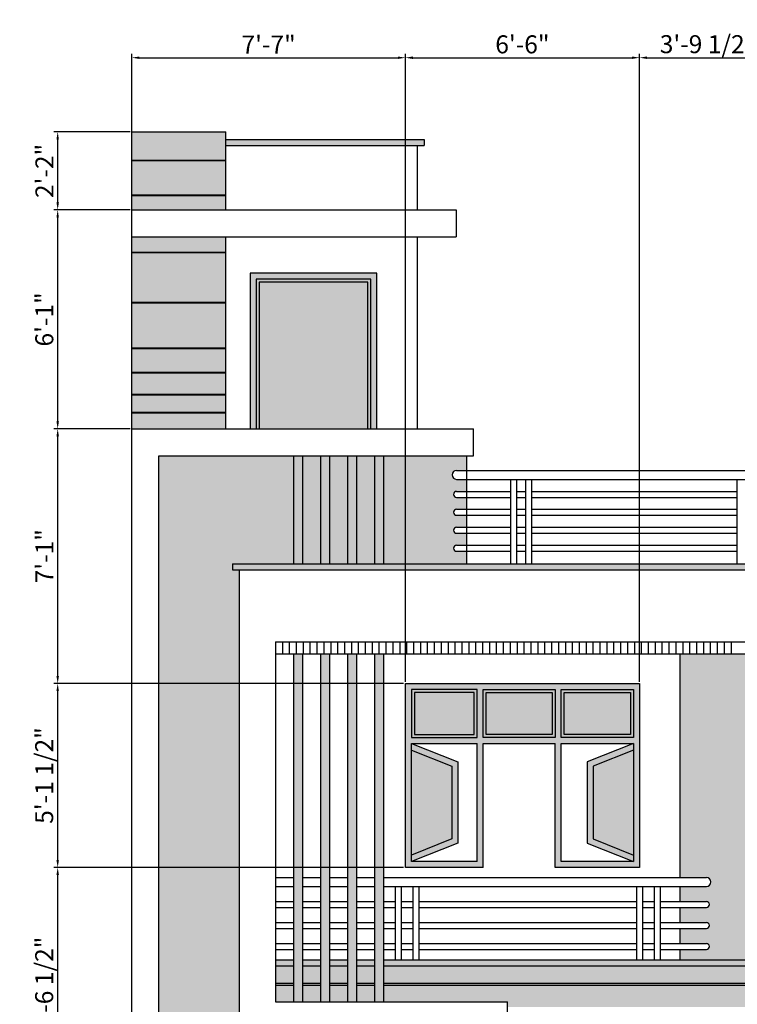
# Model space of a CAD drawing. Units: millimetres. Extents: x 4237 to 5109, y 21391 to 22486.
# Tile 2 of 17: x 4672 to 4911, y 21581 to 21909. Entities that reach past the tile are written whole.
import ezdxf

# ---------------------------------------------------------------- set-up
doc = ezdxf.new("R2010")
doc.units = ezdxf.units.MM
for name, color, linetype, lineweight in [('A-ANNO-DIMS', 2, 'Continuous', 18), ('A-ELEV', 7, 'Continuous', 25), ('A-ELEV-PATT', 252, 'Continuous', 13)]:
    doc.layers.add(name, color=color, linetype=linetype, lineweight=lineweight)
doc.styles.get("Standard").update_dxf_attribs({"font": 'arial.ttf'})
doc.dimstyles.new('ISO-25', dxfattribs={"dimtxt": 6, "dimasz": 2.5, "dimexe": 1.25, "dimexo": 0.625, "dimtad": 1, "dimdec": 1, "dimlunit": 4, "dimtxsty": 'Standard', "dimcen": 2.5, "dimadec": 0, "dimazin": 0, "dimtfac": 1, "dimtdec": 1, "dimtmove": 0, "dimatfit": 3, "dimfxl": 1, "dimarcsym": 0})

# ---------------------------------------------------------------- blocks, each defined once
blk = doc.blocks.new('*D128')
at = {"layer": 'A-ANNO-DIMS', "color": 0, "lineweight": -2, "transparency": 16777216}
for p, q in [((4709.23, 21558.46), (4709.23, 21897.84)), ((4711.73, 21896.59), (4797.95, 21896.59)), ((4800.45, 21688.54), (4800.45, 21897.84))]:
    blk.add_line(p, q, dxfattribs=at)
at = {"layer": 'A-ANNO-DIMS', "color": 0, "transparency": 16777216}
for points in [[(4711.73, 21897), (4711.73, 21896.17), (4709.23, 21896.59)], [(4797.95, 21897), (4797.95, 21896.17), (4800.45, 21896.59)]]:
    blk.add_solid(points, dxfattribs=at)
at = {"layer": 'Defpoints', "color": 0, "transparency": 16777216}
for p in [(4800.45, 21896.59), (4800.45, 21687.91), (4709.23, 21557.84)]:
    blk.add_point(p, dxfattribs=at)
at = {"layer": 'A-ANNO-DIMS', "color": 0, "transparency": 16777216, "insert": (4754.84, 21900.21), "char_height": 6, "attachment_point": 5}
blk.add_mtext('7\'-7"', dxfattribs=at)
blk = doc.blocks.new('*D129')
at = {"layer": 'A-ANNO-DIMS', "color": 0, "lineweight": -2, "transparency": 16777216}
for p, q in [((4800.45, 21688.54), (4800.45, 21897.84)), ((4802.95, 21896.59), (4876.04, 21896.59)), ((4878.54, 21688.54), (4878.54, 21897.84))]:
    blk.add_line(p, q, dxfattribs=at)
at = {"layer": 'A-ANNO-DIMS', "color": 0, "transparency": 16777216}
for points in [[(4802.95, 21897), (4802.95, 21896.17), (4800.45, 21896.59)], [(4876.04, 21897), (4876.04, 21896.17), (4878.54, 21896.59)]]:
    blk.add_solid(points, dxfattribs=at)
at = {"layer": 'Defpoints', "color": 0, "transparency": 16777216}
for p in [(4878.54, 21896.59), (4800.45, 21687.91), (4878.54, 21687.91)]:
    blk.add_point(p, dxfattribs=at)
at = {"layer": 'A-ANNO-DIMS', "color": 0, "transparency": 16777216, "insert": (4839.49, 21900.27), "char_height": 6, "attachment_point": 5}
blk.add_mtext('6\'-6"', dxfattribs=at)
blk = doc.blocks.new('*D130')
at = {"layer": 'A-ANNO-DIMS', "color": 0, "lineweight": -2, "transparency": 16777216}
for p, q in [((4878.54, 21688.54), (4878.54, 21897.84)), ((4881.04, 21896.59), (4921.78, 21896.59)), ((4924.28, 21686.68), (4924.28, 21897.84))]:
    blk.add_line(p, q, dxfattribs=at)
at = {"layer": 'A-ANNO-DIMS', "color": 0, "transparency": 16777216}
for points in [[(4881.04, 21897), (4881.04, 21896.17), (4878.54, 21896.59)], [(4921.78, 21897), (4921.78, 21896.17), (4924.28, 21896.59)]]:
    blk.add_solid(points, dxfattribs=at)
at = {"layer": 'Defpoints', "color": 0, "transparency": 16777216}
for p in [(4924.28, 21896.59), (4878.54, 21687.91), (4924.28, 21686.05)]:
    blk.add_point(p, dxfattribs=at)
at = {"layer": 'A-ANNO-DIMS', "color": 0, "transparency": 16777216, "insert": (4901.41, 21900.32), "char_height": 6, "attachment_point": 5}
blk.add_mtext('3\'-9 1/2"', dxfattribs=at)
blk = doc.blocks.new('*D140')
at = {"layer": 'A-ANNO-DIMS', "color": 0, "lineweight": -2, "transparency": 16777216}
for p, q in [((4799.82, 21626.61), (4683.23, 21626.61)), ((4684.48, 21550.76), (4684.48, 21624.11)), ((4807.6, 21548.26), (4683.23, 21548.26))]:
    blk.add_line(p, q, dxfattribs=at)
at = {"layer": 'A-ANNO-DIMS', "color": 0, "transparency": 16777216}
for points in [[(4684.06, 21624.11), (4684.89, 21624.11), (4684.48, 21626.61)], [(4684.06, 21550.76), (4684.89, 21550.76), (4684.48, 21548.26)]]:
    blk.add_solid(points, dxfattribs=at)
at = {"layer": 'Defpoints', "color": 0, "transparency": 16777216}
for p in [(4684.48, 21626.61), (4800.45, 21626.61), (4808.23, 21548.26)]:
    blk.add_point(p, dxfattribs=at)
at = {"layer": 'A-ANNO-DIMS', "color": 0, "transparency": 16777216, "insert": (4680.75, 21587.44), "char_height": 6, "attachment_point": 5, "rotation": 90}
blk.add_mtext('6\'-6 1/2"', dxfattribs=at)
blk = doc.blocks.new('*D141')
at = {"layer": 'A-ANNO-DIMS', "color": 0, "lineweight": -2, "transparency": 16777216}
for p, q in [((4799.82, 21687.91), (4683.23, 21687.91)), ((4684.48, 21629.11), (4684.48, 21685.41)), ((4799.82, 21626.61), (4683.23, 21626.61))]:
    blk.add_line(p, q, dxfattribs=at)
at = {"layer": 'A-ANNO-DIMS', "color": 0, "transparency": 16777216}
for points in [[(4684.06, 21685.41), (4684.89, 21685.41), (4684.48, 21687.91)], [(4684.06, 21629.11), (4684.89, 21629.11), (4684.48, 21626.61)]]:
    blk.add_solid(points, dxfattribs=at)
at = {"layer": 'Defpoints', "color": 0, "transparency": 16777216}
for p in [(4684.48, 21687.91), (4800.45, 21687.91), (4800.45, 21626.61)]:
    blk.add_point(p, dxfattribs=at)
at = {"layer": 'A-ANNO-DIMS', "color": 0, "transparency": 16777216, "insert": (4680.75, 21657.26), "char_height": 6, "attachment_point": 5, "rotation": 90}
blk.add_mtext('5\'-1 1/2"', dxfattribs=at)
blk = doc.blocks.new('*D142')
at = {"layer": 'A-ANNO-DIMS', "color": 0, "lineweight": -2, "transparency": 16777216}
for p, q in [((4708.6, 21772.84), (4683.23, 21772.84)), ((4684.48, 21690.41), (4684.48, 21770.34)), ((4799.82, 21687.91), (4683.23, 21687.91))]:
    blk.add_line(p, q, dxfattribs=at)
at = {"layer": 'A-ANNO-DIMS', "color": 0, "transparency": 16777216}
for points in [[(4684.06, 21770.34), (4684.89, 21770.34), (4684.48, 21772.84)], [(4684.06, 21690.41), (4684.89, 21690.41), (4684.48, 21687.91)]]:
    blk.add_solid(points, dxfattribs=at)
at = {"layer": 'Defpoints', "color": 0, "transparency": 16777216}
for p in [(4684.48, 21772.84), (4709.23, 21772.84), (4800.45, 21687.91)]:
    blk.add_point(p, dxfattribs=at)
at = {"layer": 'A-ANNO-DIMS', "color": 0, "transparency": 16777216, "insert": (4680.84, 21730.37), "char_height": 6, "attachment_point": 5, "rotation": 90}
blk.add_mtext('7\'-1"', dxfattribs=at)
blk = doc.blocks.new('*D143')
at = {"layer": 'A-ANNO-DIMS', "color": 0, "lineweight": -2, "transparency": 16777216}
for p, q in [((4708.6, 21845.84), (4683.23, 21845.84)), ((4684.48, 21775.34), (4684.48, 21843.34)), ((4708.6, 21772.84), (4683.23, 21772.84))]:
    blk.add_line(p, q, dxfattribs=at)
at = {"layer": 'A-ANNO-DIMS', "color": 0, "transparency": 16777216}
for points in [[(4684.06, 21843.34), (4684.89, 21843.34), (4684.48, 21845.84)], [(4684.06, 21775.34), (4684.89, 21775.34), (4684.48, 21772.84)]]:
    blk.add_solid(points, dxfattribs=at)
at = {"layer": 'Defpoints', "color": 0, "transparency": 16777216}
for p in [(4684.48, 21845.84), (4709.23, 21845.84), (4709.23, 21772.84)]:
    blk.add_point(p, dxfattribs=at)
at = {"layer": 'A-ANNO-DIMS', "color": 0, "transparency": 16777216, "insert": (4680.79, 21809.34), "char_height": 6, "attachment_point": 5, "rotation": 90}
blk.add_mtext('6\'-1"', dxfattribs=at)
blk = doc.blocks.new('*D144')
at = {"layer": 'A-ANNO-DIMS', "color": 0, "lineweight": -2, "transparency": 16777216}
for p, q in [((4708.6, 21871.84), (4683.23, 21871.84)), ((4684.48, 21848.34), (4684.48, 21869.34)), ((4708.6, 21845.84), (4683.23, 21845.84))]:
    blk.add_line(p, q, dxfattribs=at)
at = {"layer": 'A-ANNO-DIMS', "color": 0, "transparency": 16777216}
for points in [[(4684.06, 21869.34), (4684.89, 21869.34), (4684.48, 21871.84)], [(4684.06, 21848.34), (4684.89, 21848.34), (4684.48, 21845.84)]]:
    blk.add_solid(points, dxfattribs=at)
at = {"layer": 'Defpoints', "color": 0, "transparency": 16777216}
for p in [(4684.48, 21871.84), (4709.23, 21871.84), (4709.23, 21845.84)]:
    blk.add_point(p, dxfattribs=at)
at = {"layer": 'A-ANNO-DIMS', "color": 0, "transparency": 16777216, "insert": (4680.84, 21858.84), "char_height": 6, "attachment_point": 5, "rotation": 90}
blk.add_mtext('2\'-2"', dxfattribs=at)

msp = doc.modelspace()

# ---------------------------------------------------------------- hatches: boundary and pattern name
at = {"layer": 'A-ELEV-PATT'}
h = msp.add_hatch(color=256, dxfattribs=at)
h.dxf.hatch_style = 1
h.paths.add_polyline_path([(4740.59, 21871.84), (4709.23, 21871.84), (4709.23, 21862.48), (4740.59, 21862.48)])
h = msp.add_hatch(color=256, dxfattribs=at)
h.dxf.hatch_style = 1
h.paths.add_polyline_path([(4806.71, 21869.32), (4740.59, 21869.32), (4740.59, 21867.32), (4806.71, 21867.32)])
h = msp.add_hatch(color=256, dxfattribs=at)
h.dxf.hatch_style = 1
h.paths.add_polyline_path([(4740.59, 21862.48), (4709.23, 21862.48), (4709.23, 21862.28), (4740.59, 21862.28)])
h = msp.add_hatch(color=256, dxfattribs=at)
h.dxf.hatch_style = 1
h.paths.add_polyline_path([(4740.59, 21862.28), (4709.23, 21862.28), (4709.23, 21850.82), (4740.59, 21850.82)])
h = msp.add_hatch(color=256, dxfattribs=at)
h.dxf.hatch_style = 1
h.paths.add_polyline_path([(4740.59, 21850.82), (4709.23, 21850.82), (4709.23, 21850.62), (4740.59, 21850.62)])
h = msp.add_hatch(color=256, dxfattribs=at)
h.dxf.hatch_style = 1
h.paths.add_polyline_path([(4740.59, 21850.62), (4709.23, 21850.62), (4709.23, 21845.84), (4740.59, 21845.84)])
h = msp.add_hatch(color=256, dxfattribs=at)
h.dxf.hatch_style = 1
h.paths.add_polyline_path([(4740.59, 21836.84), (4709.23, 21836.84), (4709.23, 21831.8), (4740.59, 21831.8)])
h = msp.add_hatch(color=256, dxfattribs=at)
h.dxf.hatch_style = 1
h.paths.add_polyline_path([(4740.59, 21831.8), (4709.23, 21831.8), (4709.23, 21831.6), (4740.59, 21831.6)])
h = msp.add_hatch(color=256, dxfattribs=at)
h.dxf.hatch_style = 1
h.paths.add_polyline_path([(4740.59, 21831.6), (4709.23, 21831.6), (4709.23, 21815.08), (4740.59, 21815.08)])
h = msp.add_hatch(color=256, dxfattribs=at)
h.dxf.hatch_style = 1
h.paths.add_polyline_path([(4740.59, 21831.6), (4709.23, 21831.6), (4709.23, 21815.08), (4740.59, 21815.08)])
h = msp.add_hatch(color=256, dxfattribs=at)
h.dxf.hatch_style = 1
h.paths.add_polyline_path([(4790.91, 21824.78), (4748.66, 21824.78), (4748.66, 21772.84), (4750.66, 21772.84), (4750.66, 21822.78), (4788.91, 21822.78), (4788.91, 21772.84), (4790.91, 21772.84)])
h = msp.add_hatch(color=256, dxfattribs=at)
h.dxf.hatch_style = 1
h.paths.add_polyline_path([(4788.91, 21822.78), (4750.66, 21822.78), (4750.66, 21772.84), (4751.66, 21772.84), (4751.66, 21821.78), (4787.91, 21821.78), (4787.91, 21772.84), (4788.91, 21772.84)])
h = msp.add_hatch(color=256, dxfattribs=at)
h.dxf.hatch_style = 1
h.set_gradient(color1=(122, 175, 223), color2=(215, 235, 210), name='INVCYLINDER')
h.paths.add_polyline_path([(4787.91, 21821.78), (4751.66, 21821.78), (4751.66, 21772.84), (4787.91, 21772.84)])
h = msp.add_hatch(color=256, dxfattribs=at)
h.dxf.hatch_style = 1
h.paths.add_polyline_path([(4740.59, 21815.08), (4709.23, 21815.08), (4709.23, 21814.88), (4740.59, 21814.88)])
h = msp.add_hatch(color=256, dxfattribs=at)
h.dxf.hatch_style = 1
h.paths.add_polyline_path([(4740.59, 21814.88), (4709.23, 21814.88), (4709.23, 21799.83), (4740.59, 21799.83)])
h = msp.add_hatch(color=256, dxfattribs=at)
h.dxf.hatch_style = 1
h.paths.add_polyline_path([(4740.59, 21799.83), (4709.23, 21799.83), (4709.23, 21799.63), (4740.59, 21799.63)])
h = msp.add_hatch(color=256, dxfattribs=at)
h.dxf.hatch_style = 1
h.paths.add_polyline_path([(4740.59, 21799.63), (4709.23, 21799.63), (4709.23, 21791.76), (4740.59, 21791.76)])
h = msp.add_hatch(color=256, dxfattribs=at)
h.dxf.hatch_style = 1
h.paths.add_polyline_path([(4740.59, 21791.76), (4709.23, 21791.76), (4709.23, 21791.56), (4740.59, 21791.56)])
h = msp.add_hatch(color=256, dxfattribs=at)
h.dxf.hatch_style = 1
h.paths.add_polyline_path([(4740.59, 21791.56), (4709.23, 21791.56), (4709.23, 21784.38), (4740.59, 21784.38)])
h = msp.add_hatch(color=256, dxfattribs=at)
h.dxf.hatch_style = 1
h.paths.add_polyline_path([(4740.59, 21784.38), (4709.23, 21784.38), (4709.23, 21784.18), (4740.59, 21784.18)])
h = msp.add_hatch(color=256, dxfattribs=at)
h.dxf.hatch_style = 1
h.paths.add_polyline_path([(4740.59, 21784.18), (4709.23, 21784.18), (4709.23, 21778.39), (4740.59, 21778.39)])
h = msp.add_hatch(color=256, dxfattribs=at)
h.dxf.hatch_style = 1
h.paths.add_polyline_path([(4740.59, 21778.39), (4709.23, 21778.39), (4709.23, 21778.19), (4740.59, 21778.19)])
h = msp.add_hatch(color=256, dxfattribs=at)
h.dxf.hatch_style = 1
h.paths.add_polyline_path([(4740.59, 21778.19), (4709.23, 21778.19), (4709.23, 21772.84), (4740.59, 21772.84)])
h = msp.add_hatch(color=256, dxfattribs=at)
h.dxf.hatch_style = 1
h.paths.add_polyline_path([(4763.12, 21763.84), (4718.23, 21763.84), (4718.23, 21557.84), (4745.15, 21557.84), (4745.15, 21725.84), (4742.84, 21725.84), (4742.84, 21727.84), (4763.12, 21727.84)])
h = msp.add_hatch(color=256, dxfattribs=at)
h.dxf.hatch_style = 1
h.paths.add_polyline_path([(4766.12, 21763.84), (4763.12, 21763.84), (4763.12, 21727.84), (4766.12, 21727.84)])
h = msp.add_hatch(color=256, dxfattribs=at)
h.dxf.hatch_style = 1
h.paths.add_polyline_path([(4772.12, 21763.84), (4766.12, 21763.84), (4766.12, 21727.84), (4772.12, 21727.84)])
h = msp.add_hatch(color=256, dxfattribs=at)
h.dxf.hatch_style = 1
h.paths.add_polyline_path([(4775.12, 21763.84), (4772.12, 21763.84), (4772.12, 21727.84), (4775.12, 21727.84)])
h = msp.add_hatch(color=256, dxfattribs=at)
h.dxf.hatch_style = 1
h.paths.add_polyline_path([(4781.12, 21763.84), (4775.12, 21763.84), (4775.12, 21727.84), (4781.12, 21727.84)])
h = msp.add_hatch(color=256, dxfattribs=at)
h.dxf.hatch_style = 1
h.paths.add_polyline_path([(4784.12, 21763.84), (4781.12, 21763.84), (4781.12, 21727.84), (4784.12, 21727.84)])
h = msp.add_hatch(color=256, dxfattribs=at)
h.dxf.hatch_style = 1
h.paths.add_polyline_path([(4790.12, 21763.84), (4784.12, 21763.84), (4784.12, 21727.84), (4790.12, 21727.84)])
h = msp.add_hatch(color=256, dxfattribs=at)
h.dxf.hatch_style = 1
h.paths.add_polyline_path([(4793.12, 21763.84), (4790.12, 21763.84), (4790.12, 21727.84), (4793.12, 21727.84)])
h = msp.add_hatch(color=256, dxfattribs=at)
h.dxf.hatch_style = 1
h.paths.add_polyline_path([(4817.54, 21740.01), (4820.82, 21740.01), (4820.82, 21744.01), (4817.54, 21744.01, -1), (4817.54, 21746.01), (4820.82, 21746.01), (4820.82, 21750.01), (4817.54, 21750.01, -1), (4817.54, 21752.01), (4820.82, 21752.01), (4820.82, 21756.01), (4817.54, 21756.01, -1), (4817.54, 21759.01), (4820.82, 21759.01), (4820.82, 21763.84), (4793.12, 21763.84), (4793.12, 21727.84), (4820.82, 21727.84), (4820.82, 21732.01), (4817.54, 21732.01, -1), (4817.54, 21734.01), (4820.82, 21734.01), (4820.82, 21738.01), (4817.54, 21738.01, -1)])
h = msp.add_hatch(color=256, dxfattribs=at)
h.dxf.hatch_style = 1
h.paths.add_polyline_path([(5017.14, 21727.84), (4742.84, 21727.84), (4742.84, 21725.84), (5017.14, 21725.84)])
h = msp.add_hatch(color=256, dxfattribs=at)
h.dxf.hatch_style = 1
h.paths.add_polyline_path([(4766.12, 21697.84), (4763.12, 21697.84), (4763.12, 21581.84), (4766.12, 21581.84)])
h = msp.add_hatch(color=256, dxfattribs=at)
h.dxf.hatch_style = 1
h.paths.add_polyline_path([(4775.12, 21697.84), (4772.12, 21697.84), (4772.12, 21581.84), (4775.12, 21581.84)])
h = msp.add_hatch(color=256, dxfattribs=at)
h.dxf.hatch_style = 1
h.paths.add_polyline_path([(4784.12, 21697.84), (4781.12, 21697.84), (4781.12, 21581.84), (4784.12, 21581.84)])
h = msp.add_hatch(color=256, dxfattribs=at)
h.dxf.hatch_style = 1
h.paths.add_polyline_path([(4793.12, 21697.84), (4790.12, 21697.84), (4790.12, 21581.84), (4793.12, 21581.84)])
h = msp.add_hatch(color=256, dxfattribs=at)
h.dxf.hatch_style = 1
h.paths.add_polyline_path([(4978.93, 21697.84), (4892.07, 21697.84), (4892.07, 21623.26), (4900.89, 21623.26, -1), (4900.89, 21620.26), (4892.07, 21620.26), (4892.07, 21615.26), (4900.89, 21615.26, -1), (4900.89, 21613.26), (4892.07, 21613.26), (4892.07, 21608.26), (4900.89, 21608.26, -1), (4900.89, 21606.26), (4892.07, 21606.26), (4892.07, 21601.26), (4900.89, 21601.26, -1), (4900.89, 21599.26), (4892.07, 21599.26), (4892.07, 21595.84), (4978.93, 21595.84)])
h.paths.add_polyline_path([(4924.28, 21686.05), (4966.23, 21686.05), (4966.23, 21613.83), (4924.28, 21613.83)], flags=16)
h.paths.add_polyline_path([(4926.28, 21661.68), (4940.28, 21661.68), (4940.28, 21615.68), (4926.28, 21615.68)], flags=0)
h.paths.add_polyline_path([(4942.28, 21661.68), (4964.23, 21661.68), (4964.23, 21615.68), (4942.28, 21615.68)], flags=0)
h.paths.add_polyline_path([(4926.28, 21663.68), (4926.28, 21684.05), (4964.23, 21684.05), (4964.23, 21663.68)], flags=0)
h.paths.add_polyline_path([(4927.28, 21664.68), (4927.28, 21683.05), (4963.23, 21683.05), (4963.23, 21664.68)], flags=0)
h = msp.add_hatch(color=256, dxfattribs=at)
h.dxf.hatch_style = 1
h.paths.add_polyline_path([(4826.45, 21667.91), (4850.45, 21667.91), (4850.45, 21626.61), (4878.54, 21626.61), (4878.54, 21687.91), (4800.45, 21687.91), (4800.45, 21626.61), (4826.45, 21626.61)])
h.paths.add_polyline_path([(4802.45, 21628.61), (4802.45, 21667.91), (4824.45, 21667.91), (4824.45, 21628.61)], flags=16)
h.paths.add_polyline_path([(4802.45, 21669.91), (4802.45, 21685.91), (4824.45, 21685.91), (4824.45, 21669.91)], flags=16)
h.paths.add_polyline_path([(4803.45, 21670.91), (4803.45, 21684.91), (4823.45, 21684.91), (4823.45, 21670.91)], flags=0)
h.paths.add_polyline_path([(4826.45, 21669.91), (4826.45, 21685.91), (4850.45, 21685.91), (4850.45, 21669.91)], flags=16)
h.paths.add_polyline_path([(4827.45, 21670.91), (4827.45, 21684.91), (4849.45, 21684.91), (4849.45, 21670.91)], flags=0)
h.paths.add_polyline_path([(4852.45, 21628.61), (4852.45, 21667.91), (4876.54, 21667.91), (4876.54, 21628.61)], flags=16)
h.paths.add_polyline_path([(4852.45, 21669.91), (4852.45, 21685.91), (4876.54, 21685.91), (4876.54, 21669.91)], flags=16)
h.paths.add_polyline_path([(4853.45, 21670.91), (4853.45, 21684.91), (4875.54, 21684.91), (4875.54, 21670.91)], flags=0)
h = msp.add_hatch(color=256, dxfattribs=at)
h.dxf.hatch_style = 1
h.set_gradient(color1=(122, 175, 223), color2=(215, 235, 210), name='CYLINDER')
h.paths.add_polyline_path([(4824.45, 21685.91), (4802.45, 21685.91), (4802.45, 21669.91), (4824.45, 21669.91)])
h.paths.add_polyline_path([(4823.45, 21684.91), (4823.45, 21670.91), (4803.45, 21670.91), (4803.45, 21684.91)], flags=16)
h = msp.add_hatch(color=256, dxfattribs=at)
h.dxf.hatch_style = 1
h.set_gradient(color1=(122, 175, 223), color2=(215, 235, 210), name='HEMISPHERICAL')
h.paths.add_polyline_path([(4823.45, 21684.91), (4803.45, 21684.91), (4803.45, 21670.91), (4823.45, 21670.91)])
h = msp.add_hatch(color=256, dxfattribs=at)
h.dxf.hatch_style = 1
h.set_gradient(color1=(122, 175, 223), color2=(215, 235, 210), name='CYLINDER')
h.paths.add_polyline_path([(4850.45, 21685.91), (4826.45, 21685.91), (4826.45, 21669.91), (4850.45, 21669.91)])
h.paths.add_polyline_path([(4849.45, 21684.91), (4849.45, 21670.91), (4827.45, 21670.91), (4827.45, 21684.91)], flags=16)
h = msp.add_hatch(color=256, dxfattribs=at)
h.dxf.hatch_style = 1
h.set_gradient(color1=(122, 175, 223), color2=(215, 235, 210), name='HEMISPHERICAL')
h.paths.add_polyline_path([(4849.45, 21684.91), (4827.45, 21684.91), (4827.45, 21670.91), (4849.45, 21670.91)])
h = msp.add_hatch(color=256, dxfattribs=at)
h.dxf.hatch_style = 1
h.set_gradient(color1=(122, 175, 223), color2=(215, 235, 210), name='CYLINDER')
h.paths.add_polyline_path([(4876.54, 21685.91), (4852.45, 21685.91), (4852.45, 21669.91), (4876.54, 21669.91)])
h.paths.add_polyline_path([(4875.54, 21684.91), (4875.54, 21670.91), (4853.45, 21670.91), (4853.45, 21684.91)], flags=16)
h = msp.add_hatch(color=256, dxfattribs=at)
h.dxf.hatch_style = 1
h.set_gradient(color1=(122, 175, 223), color2=(215, 235, 210), name='HEMISPHERICAL')
h.paths.add_polyline_path([(4875.54, 21684.91), (4853.45, 21684.91), (4853.45, 21670.91), (4875.54, 21670.91)])
h = msp.add_hatch(color=256, dxfattribs=at)
h.dxf.hatch_style = 1
h.paths.add_polyline_path([(4817.91, 21661.78), (4802.45, 21667.91), (4802.45, 21665.76), (4815.91, 21660.43), (4815.91, 21636.1), (4802.45, 21630.76), (4802.45, 21628.61), (4817.91, 21634.74)])
h = msp.add_hatch(color=256, dxfattribs=at)
h.dxf.hatch_style = 1
h.paths.add_polyline_path([(4863.07, 21660.43), (4876.54, 21665.76), (4876.54, 21667.91), (4861.07, 21661.78), (4861.07, 21634.74), (4876.54, 21628.61), (4876.54, 21630.76), (4863.07, 21636.1)])
h = msp.add_hatch(color=256, dxfattribs=at)
h.dxf.hatch_style = 1
h.set_gradient(color1=(122, 175, 223), color2=(215, 235, 210), name='CYLINDER')
h.paths.add_polyline_path([(4815.91, 21660.43), (4802.45, 21665.76), (4802.45, 21630.76), (4815.91, 21636.1)])
h = msp.add_hatch(color=256, dxfattribs=at)
h.dxf.hatch_style = 1
h.set_gradient(color1=(122, 175, 223), color2=(215, 235, 210), name='CYLINDER')
h.paths.add_polyline_path([(4876.54, 21665.76), (4863.07, 21660.43), (4863.07, 21636.1), (4876.54, 21630.76)])
h = msp.add_hatch(color=256, dxfattribs=at)
h.dxf.hatch_style = 1
h.paths.add_polyline_path([(5033.17, 21598.15), (5022.76, 21598.15), (5022.76, 21595.84), (5025.55, 21595.84), (5025.55, 21593.84), (4991.17, 21593.84), (4991.17, 21595.84), (4997.2, 21595.84), (4997.2, 21598.15), (4978.93, 21598.15), (4978.93, 21595.84), (4981.84, 21595.84), (4981.84, 21593.84), (4793.12, 21593.84), (4793.12, 21588.01), (5033.17, 21588.01)])
h = msp.add_hatch(color=256, dxfattribs=at)
h.dxf.hatch_style = 1
h.paths.add_polyline_path([(4763.12, 21595.84), (4757.12, 21595.84), (4757.12, 21593.84), (4763.12, 21593.84)])
h = msp.add_hatch(color=256, dxfattribs=at)
h.dxf.hatch_style = 1
h.paths.add_polyline_path([(4772.12, 21595.84), (4766.12, 21595.84), (4766.12, 21593.84), (4772.12, 21593.84)])
h = msp.add_hatch(color=256, dxfattribs=at)
h.dxf.hatch_style = 1
h.paths.add_polyline_path([(4781.12, 21595.84), (4775.12, 21595.84), (4775.12, 21593.84), (4781.12, 21593.84)])
h = msp.add_hatch(color=256, dxfattribs=at)
h.dxf.hatch_style = 1
h.paths.add_polyline_path([(4790.12, 21595.84), (4784.12, 21595.84), (4784.12, 21593.84), (4790.12, 21593.84)])
h = msp.add_hatch(color=256, dxfattribs=at)
h.dxf.hatch_style = 1
h.paths.add_polyline_path([(4981.84, 21595.84), (4793.12, 21595.84), (4793.12, 21593.84), (4981.84, 21593.84)])
h = msp.add_hatch(color=256, dxfattribs=at)
h.dxf.hatch_style = 1
h.paths.add_polyline_path([(4763.12, 21593.84), (4757.12, 21593.84), (4757.12, 21588.01), (4763.12, 21588.01)])
h = msp.add_hatch(color=256, dxfattribs=at)
h.dxf.hatch_style = 1
h.paths.add_polyline_path([(4772.12, 21593.84), (4766.12, 21593.84), (4766.12, 21588.01), (4772.12, 21588.01)])
h = msp.add_hatch(color=256, dxfattribs=at)
h.dxf.hatch_style = 1
h.paths.add_polyline_path([(4781.12, 21593.84), (4775.12, 21593.84), (4775.12, 21588.01), (4781.12, 21588.01)])
h = msp.add_hatch(color=256, dxfattribs=at)
h.dxf.hatch_style = 1
h.paths.add_polyline_path([(4790.12, 21593.84), (4784.12, 21593.84), (4784.12, 21588.01), (4790.12, 21588.01)])
h = msp.add_hatch(color=256, dxfattribs=at)
h.dxf.hatch_style = 1
h.paths.add_polyline_path([(4763.12, 21588.01), (4757.12, 21588.01), (4757.12, 21587.38), (4763.12, 21587.38)])
h = msp.add_hatch(color=256, dxfattribs=at)
h.dxf.hatch_style = 1
h.paths.add_polyline_path([(4772.12, 21588.01), (4766.12, 21588.01), (4766.12, 21587.38), (4772.12, 21587.38)])
h = msp.add_hatch(color=256, dxfattribs=at)
h.dxf.hatch_style = 1
h.paths.add_polyline_path([(4781.12, 21588.01), (4775.12, 21588.01), (4775.12, 21587.38), (4781.12, 21587.38)])
h = msp.add_hatch(color=256, dxfattribs=at)
h.dxf.hatch_style = 1
h.paths.add_polyline_path([(4790.12, 21588.01), (4784.12, 21588.01), (4784.12, 21587.38), (4790.12, 21587.38)])
h = msp.add_hatch(color=256, dxfattribs=at)
h.dxf.hatch_style = 1
h.paths.add_polyline_path([(5033.17, 21588.01), (4793.12, 21588.01), (4793.12, 21587.38), (5033.17, 21587.38)])
h = msp.add_hatch(color=256, dxfattribs=at)
h.dxf.hatch_style = 1
h.paths.add_polyline_path([(4763.12, 21587.38), (4757.12, 21587.38), (4757.12, 21581.84), (4763.12, 21581.84)])
h = msp.add_hatch(color=256, dxfattribs=at)
h.dxf.hatch_style = 1
h.paths.add_polyline_path([(4772.12, 21587.38), (4766.12, 21587.38), (4766.12, 21581.84), (4772.12, 21581.84)])
h = msp.add_hatch(color=256, dxfattribs=at)
h.dxf.hatch_style = 1
h.paths.add_polyline_path([(4781.12, 21587.38), (4775.12, 21587.38), (4775.12, 21581.84), (4781.12, 21581.84)])
h = msp.add_hatch(color=256, dxfattribs=at)
h.dxf.hatch_style = 1
h.paths.add_polyline_path([(4790.12, 21587.38), (4784.12, 21587.38), (4784.12, 21581.84), (4790.12, 21581.84)])
h = msp.add_hatch(color=256, dxfattribs=at)
h.dxf.hatch_style = 1
h.paths.add_polyline_path([(5033.17, 21587.38), (4793.12, 21587.38), (4793.12, 21581.84), (4834.56, 21581.84), (4834.56, 21580.12), (5033.17, 21580.12)])

# ---------------------------------------------------------------- linework, layer by layer
at = {"layer": 'A-ELEV'}
for p, q in [((4709.23, 21425.84), (4709.23, 21871.84)), ((4709.23, 21871.84), (4740.59, 21871.84)), ((4740.59, 21845.84), (4740.59, 21871.84)), ((4740.59, 21869.32), (4806.71, 21869.32)), ((4740.59, 21867.32), (4806.71, 21867.32)), ((4804.53, 21845.84), (4804.53, 21867.32)), ((4806.71, 21869.32), (4806.71, 21867.32)), ((4709.23, 21862.48), (4740.59, 21862.48)), ((4709.23, 21862.28), (4740.59, 21862.28)), ((4709.23, 21850.82), (4740.59, 21850.82)), ((4709.23, 21850.62), (4740.59, 21850.62)), ((4709.23, 21845.84), (4817.34, 21845.84)), ((4817.34, 21845.84), (4817.34, 21836.84)), ((4709.23, 21836.84), (4817.34, 21836.84)), ((4740.59, 21772.84), (4740.59, 21836.84)), ((4804.53, 21772.84), (4804.53, 21836.84)), ((4709.23, 21831.8), (4740.59, 21831.8)), ((4709.23, 21831.6), (4740.59, 21831.6)), ((4709.23, 21815.08), (4740.59, 21815.08)), ((4709.23, 21814.88), (4740.59, 21814.88)), ((4709.23, 21799.83), (4740.59, 21799.83)), ((4709.23, 21799.63), (4740.59, 21799.63)), ((4709.23, 21791.76), (4740.59, 21791.76)), ((4709.23, 21791.56), (4740.59, 21791.56)), ((4709.23, 21784.38), (4740.59, 21784.38)), ((4709.23, 21784.18), (4740.59, 21784.18)), ((4709.23, 21778.39), (4740.59, 21778.39)), ((4709.23, 21778.19), (4740.59, 21778.19)), ((4709.23, 21772.84), (4823.22, 21772.84)), ((4823.22, 21763.84), (4823.22, 21772.84)), ((4718.23, 21557.84), (4718.23, 21763.84)), ((4718.23, 21763.84), (4823.22, 21763.84)), ((4763.12, 21763.84), (4763.12, 21727.84)), ((4766.12, 21763.84), (4766.12, 21727.84)), ((4772.12, 21763.84), (4772.12, 21727.84)), ((4775.12, 21763.84), (4775.12, 21727.84)), ((4781.12, 21763.84), (4781.12, 21727.84)), ((4784.12, 21763.84), (4784.12, 21727.84)), ((4790.12, 21763.84), (4790.12, 21727.84)), ((4793.12, 21763.84), (4793.12, 21727.84)), ((4820.82, 21763.84), (4820.82, 21727.84)), ((4817.54, 21759.01), (4931.32, 21759.01)), ((4817.54, 21756.01), (4931.32, 21756.01)), ((4835.52, 21756.01), (4835.52, 21727.84)), ((4837.52, 21756.01), (4837.52, 21727.84)), ((4840.56, 21756.01), (4840.56, 21727.84)), ((4842.56, 21756.01), (4842.56, 21727.84)), ((4910.97, 21756.01), (4910.97, 21727.84)), ((4817.54, 21752.01), (4835.52, 21752.01)), ((4817.54, 21750.01), (4835.52, 21750.01)), ((4837.52, 21752.01), (4840.56, 21752.01)), ((4837.52, 21750.01), (4840.56, 21750.01)), ((4842.56, 21752.01), (4910.97, 21752.01)), ((4842.56, 21750.01), (4910.97, 21750.01)), ((4817.54, 21746.01), (4835.52, 21746.01)), ((4837.52, 21746.01), (4840.56, 21746.01)), ((4842.56, 21746.01), (4910.97, 21746.01)), ((4817.54, 21744.01), (4835.52, 21744.01)), ((4837.52, 21744.01), (4840.56, 21744.01)), ((4842.56, 21744.01), (4910.97, 21744.01)), ((4817.54, 21740.01), (4835.52, 21740.01)), ((4837.52, 21740.01), (4840.56, 21740.01)), ((4842.56, 21740.01), (4910.97, 21740.01)), ((4817.54, 21738.01), (4835.52, 21738.01)), ((4837.52, 21738.01), (4840.56, 21738.01)), ((4842.56, 21738.01), (4910.97, 21738.01)), ((4817.54, 21734.01), (4835.52, 21734.01)), ((4837.52, 21734.01), (4840.56, 21734.01)), ((4842.56, 21734.01), (4910.97, 21734.01)), ((4817.54, 21732.01), (4835.52, 21732.01)), ((4837.52, 21732.01), (4840.56, 21732.01)), ((4842.56, 21732.01), (4910.97, 21732.01)), ((4742.84, 21727.84), (5017.14, 21727.84)), ((4742.84, 21727.84), (4742.84, 21725.84)), ((4742.84, 21725.84), (5017.14, 21725.84)), ((4745.15, 21557.84), (4745.15, 21725.84)), ((4757.12, 21701.84), (5017.14, 21701.84)), ((4757.12, 21701.84), (4757.12, 21581.84)), ((4759.42, 21701.84), (4759.42, 21697.84)), ((4761.72, 21701.84), (4761.72, 21697.84)), ((4764.02, 21701.84), (4764.02, 21697.84)), ((4766.33, 21701.84), (4766.33, 21697.84)), ((4768.63, 21701.84), (4768.63, 21697.84)), ((4770.93, 21701.84), (4770.93, 21697.84)), ((4773.23, 21701.84), (4773.23, 21697.84)), ((4775.54, 21701.84), (4775.54, 21697.84)), ((4777.84, 21701.84), (4777.84, 21697.84)), ((4780.14, 21701.84), (4780.14, 21697.84)), ((4782.44, 21701.84), (4782.44, 21697.84)), ((4784.75, 21701.84), (4784.75, 21697.84)), ((4787.05, 21701.84), (4787.05, 21697.84)), ((4789.35, 21701.84), (4789.35, 21697.84)), ((4791.65, 21701.84), (4791.65, 21697.84)), ((4793.96, 21701.84), (4793.96, 21697.84)), ((4796.26, 21701.84), (4796.26, 21697.84)), ((4798.56, 21701.84), (4798.56, 21697.84)), ((4800.86, 21701.84), (4800.86, 21697.84)), ((4803.16, 21701.84), (4803.16, 21697.84)), ((4805.47, 21701.84), (4805.47, 21697.84)), ((4807.77, 21701.84), (4807.77, 21697.84)), ((4810.07, 21701.84), (4810.07, 21697.84)), ((4812.37, 21701.84), (4812.37, 21697.84)), ((4814.68, 21701.84), (4814.68, 21697.84)), ((4816.98, 21701.84), (4816.98, 21697.84)), ((4819.28, 21701.84), (4819.28, 21697.84)), ((4821.58, 21701.84), (4821.58, 21697.84)), ((4823.89, 21701.84), (4823.89, 21697.84)), ((4826.19, 21701.84), (4826.19, 21697.84)), ((4828.49, 21701.84), (4828.49, 21697.84)), ((4830.79, 21701.84), (4830.79, 21697.84)), ((4833.1, 21701.84), (4833.1, 21697.84)), ((4835.4, 21701.84), (4835.4, 21697.84)), ((4837.7, 21701.84), (4837.7, 21697.84)), ((4840, 21701.84), (4840, 21697.84)), ((4842.31, 21701.84), (4842.31, 21697.84)), ((4844.61, 21701.84), (4844.61, 21697.84)), ((4846.91, 21701.84), (4846.91, 21697.84)), ((4849.21, 21701.84), (4849.21, 21697.84)), ((4851.51, 21701.84), (4851.51, 21697.84)), ((4853.82, 21701.84), (4853.82, 21697.84)), ((4856.12, 21701.84), (4856.12, 21697.84)), ((4858.42, 21701.84), (4858.42, 21697.84)), ((4860.72, 21701.84), (4860.72, 21697.84)), ((4863.03, 21701.84), (4863.03, 21697.84)), ((4865.33, 21701.84), (4865.33, 21697.84)), ((4867.63, 21701.84), (4867.63, 21697.84)), ((4869.93, 21701.84), (4869.93, 21697.84)), ((4872.24, 21701.84), (4872.24, 21697.84)), ((4874.54, 21701.84), (4874.54, 21697.84)), ((4876.84, 21701.84), (4876.84, 21697.84)), ((4879.14, 21701.84), (4879.14, 21697.84)), ((4881.45, 21701.84), (4881.45, 21697.84)), ((4883.75, 21701.84), (4883.75, 21697.84)), ((4886.05, 21701.84), (4886.05, 21697.84)), ((4888.35, 21701.84), (4888.35, 21697.84)), ((4890.66, 21701.84), (4890.66, 21697.84)), ((4892.96, 21701.84), (4892.96, 21697.84)), ((4895.26, 21701.84), (4895.26, 21697.84)), ((4897.56, 21701.84), (4897.56, 21697.84)), ((4899.86, 21701.84), (4899.86, 21697.84)), ((4902.17, 21701.84), (4902.17, 21697.84)), ((4904.47, 21701.84), (4904.47, 21697.84)), ((4906.77, 21701.84), (4906.77, 21697.84)), ((4909.07, 21701.84), (4909.07, 21697.84)), ((4757.12, 21697.84), (5013.1, 21697.84)), ((4763.12, 21697.84), (4763.12, 21581.84)), ((4766.12, 21697.84), (4766.12, 21581.84)), ((4772.12, 21697.84), (4772.12, 21581.84)), ((4775.12, 21697.84), (4775.12, 21581.84)), ((4781.12, 21697.84), (4781.12, 21581.84)), ((4784.12, 21697.84), (4784.12, 21581.84)), ((4790.12, 21697.84), (4790.12, 21581.84)), ((4793.12, 21697.84), (4793.12, 21581.84)), ((4892.07, 21623.26), (4892.07, 21697.84)), ((4800.45, 21687.91), (4878.54, 21687.91)), ((4800.45, 21626.61), (4800.45, 21687.91)), ((4878.54, 21687.91), (4878.54, 21626.61)), ((4802.45, 21667.91), (4824.45, 21667.91)), ((4802.45, 21628.61), (4802.45, 21667.91)), ((4824.45, 21628.61), (4824.45, 21667.91)), ((4826.45, 21667.91), (4850.45, 21667.91)), ((4826.45, 21626.61), (4826.45, 21667.91)), ((4850.45, 21626.61), (4850.45, 21667.91)), ((4852.45, 21667.91), (4876.54, 21667.91)), ((4852.45, 21628.61), (4852.45, 21667.91)), ((4876.54, 21667.91), (4876.54, 21628.61)), ((4824.45, 21628.61), (4802.45, 21628.61)), ((4876.54, 21628.61), (4852.45, 21628.61)), ((4826.45, 21626.61), (4800.45, 21626.61)), ((4878.54, 21626.61), (4850.45, 21626.61)), ((4757.12, 21623.26), (4763.12, 21623.26)), ((4766.12, 21623.26), (4772.12, 21623.26)), ((4775.12, 21623.26), (4781.12, 21623.26)), ((4784.12, 21623.26), (4790.12, 21623.26)), ((4793.12, 21623.26), (4900.89, 21623.26)), ((4757.12, 21620.26), (4763.12, 21620.26)), ((4766.12, 21620.26), (4772.12, 21620.26)), ((4775.12, 21620.26), (4781.12, 21620.26)), ((4784.12, 21620.26), (4790.12, 21620.26)), ((4793.12, 21620.26), (4900.89, 21620.26)), ((4797.03, 21620.26), (4797.03, 21595.84)), ((4799.03, 21620.26), (4799.03, 21595.84)), ((4802.94, 21620.26), (4802.94, 21595.84)), ((4804.94, 21620.26), (4804.94, 21595.84)), ((4877.51, 21620.26), (4877.51, 21595.84)), ((4879.51, 21620.26), (4879.51, 21595.84)), ((4883.42, 21620.26), (4883.42, 21595.84)), ((4885.42, 21620.26), (4885.42, 21595.84)), ((4892.07, 21615.26), (4892.07, 21620.26)), ((4757.12, 21615.26), (4763.12, 21615.26)), ((4766.12, 21615.26), (4772.12, 21615.26)), ((4775.12, 21615.26), (4781.12, 21615.26)), ((4784.12, 21615.26), (4790.12, 21615.26)), ((4793.12, 21615.26), (4797.03, 21615.26)), ((4799.03, 21615.26), (4802.94, 21615.26)), ((4804.94, 21615.26), (4877.51, 21615.26)), ((4879.51, 21615.26), (4883.42, 21615.26)), ((4885.42, 21615.26), (4900.89, 21615.26)), ((4757.12, 21613.26), (4763.12, 21613.26)), ((4766.12, 21613.26), (4772.12, 21613.26)), ((4775.12, 21613.26), (4781.12, 21613.26)), ((4784.12, 21613.26), (4790.12, 21613.26)), ((4793.12, 21613.26), (4797.03, 21613.26)), ((4799.03, 21613.26), (4802.94, 21613.26)), ((4804.94, 21613.26), (4877.51, 21613.26)), ((4879.51, 21613.26), (4883.42, 21613.26)), ((4885.42, 21613.26), (4900.89, 21613.26)), ((4892.07, 21608.26), (4892.07, 21613.26)), ((4757.12, 21608.26), (4763.12, 21608.26)), ((4766.12, 21608.26), (4772.12, 21608.26)), ((4775.12, 21608.26), (4781.12, 21608.26)), ((4784.12, 21608.26), (4790.12, 21608.26)), ((4793.12, 21608.26), (4797.03, 21608.26)), ((4799.03, 21608.26), (4802.94, 21608.26)), ((4804.94, 21608.26), (4877.51, 21608.26)), ((4879.51, 21608.26), (4883.42, 21608.26)), ((4885.42, 21608.26), (4900.89, 21608.26)), ((4757.12, 21606.26), (4763.12, 21606.26)), ((4766.12, 21606.26), (4772.12, 21606.26)), ((4775.12, 21606.26), (4781.12, 21606.26)), ((4784.12, 21606.26), (4790.12, 21606.26)), ((4793.12, 21606.26), (4797.03, 21606.26)), ((4799.03, 21606.26), (4802.94, 21606.26)), ((4804.94, 21606.26), (4877.51, 21606.26)), ((4879.51, 21606.26), (4883.42, 21606.26)), ((4885.42, 21606.26), (4900.89, 21606.26)), ((4892.07, 21601.26), (4892.07, 21606.26)), ((4757.12, 21601.26), (4763.12, 21601.26)), ((4766.12, 21601.26), (4772.12, 21601.26)), ((4775.12, 21601.26), (4781.12, 21601.26)), ((4784.12, 21601.26), (4790.12, 21601.26)), ((4793.12, 21601.26), (4797.03, 21601.26)), ((4799.03, 21601.26), (4802.94, 21601.26)), ((4804.94, 21601.26), (4877.51, 21601.26)), ((4879.51, 21601.26), (4883.42, 21601.26)), ((4885.42, 21601.26), (4900.89, 21601.26)), ((4757.12, 21599.26), (4763.12, 21599.26)), ((4766.12, 21599.26), (4772.12, 21599.26)), ((4775.12, 21599.26), (4781.12, 21599.26)), ((4784.12, 21599.26), (4790.12, 21599.26)), ((4793.12, 21599.26), (4797.03, 21599.26)), ((4799.03, 21599.26), (4802.94, 21599.26)), ((4804.94, 21599.26), (4877.51, 21599.26)), ((4879.51, 21599.26), (4883.42, 21599.26)), ((4885.42, 21599.26), (4900.89, 21599.26)), ((4892.07, 21595.84), (4892.07, 21599.26)), ((4757.12, 21595.84), (4763.12, 21595.84)), ((4766.12, 21595.84), (4772.12, 21595.84)), ((4775.12, 21595.84), (4781.12, 21595.84)), ((4784.12, 21595.84), (4790.12, 21595.84)), ((4793.12, 21595.84), (4981.84, 21595.84)), ((4757.12, 21593.84), (4763.12, 21593.84)), ((4766.12, 21593.84), (4772.12, 21593.84)), ((4775.12, 21593.84), (4781.12, 21593.84)), ((4784.12, 21593.84), (4790.12, 21593.84)), ((4793.12, 21593.84), (4981.84, 21593.84)), ((4757.12, 21588.01), (4763.12, 21588.01)), ((4766.12, 21588.01), (4772.12, 21588.01)), ((4775.12, 21588.01), (4781.12, 21588.01)), ((4784.12, 21588.01), (4790.12, 21588.01)), ((4793.12, 21588.01), (5033.17, 21588.01)), ((4757.12, 21587.38), (4763.12, 21587.38)), ((4766.12, 21587.38), (4772.12, 21587.38)), ((4775.12, 21587.38), (4781.12, 21587.38)), ((4784.12, 21587.38), (4790.12, 21587.38)), ((4793.12, 21587.38), (5033.17, 21587.38)), ((4757.12, 21581.84), (4834.56, 21581.84)), ((4834.56, 21557.84), (4834.56, 21581.84))]:
    msp.add_line(p, q, dxfattribs=at)
for points in [[(4790.91, 21772.84), (4790.91, 21824.78), (4748.66, 21824.78), (4748.66, 21772.84)], [(4788.91, 21772.84), (4788.91, 21822.78), (4750.66, 21822.78), (4750.66, 21772.84)], [(4787.91, 21772.84), (4787.91, 21821.78), (4751.66, 21821.78), (4751.66, 21772.84)], [(4802.45, 21667.91), (4817.91, 21661.78), (4817.91, 21634.74), (4802.45, 21628.61)], [(4876.54, 21667.91), (4861.07, 21661.78), (4861.07, 21634.74), (4876.54, 21628.61)], [(4802.45, 21665.76), (4815.91, 21660.43), (4815.91, 21636.1), (4802.45, 21630.76)], [(4876.54, 21665.76), (4863.07, 21660.43), (4863.07, 21636.1), (4876.54, 21630.76)]]:
    msp.add_lwpolyline(points, dxfattribs=at)
for points in [[(4802.45, 21685.91), (4802.45, 21669.91), (4824.45, 21669.91), (4824.45, 21685.91)], [(4803.45, 21684.91), (4803.45, 21670.91), (4823.45, 21670.91), (4823.45, 21684.91)], [(4850.45, 21669.91), (4826.45, 21669.91), (4826.45, 21685.91), (4850.45, 21685.91)], [(4849.45, 21670.91), (4827.45, 21670.91), (4827.45, 21684.91), (4849.45, 21684.91)], [(4876.54, 21669.91), (4852.45, 21669.91), (4852.45, 21685.91), (4876.54, 21685.91)], [(4875.54, 21670.91), (4853.45, 21670.91), (4853.45, 21684.91), (4875.54, 21684.91)]]:
    msp.add_lwpolyline(points, close=True, dxfattribs=at)
for centre, radius, start, end in [((4817.54, 21757.51), 1.5, 90, 270), ((4817.54, 21751.01), 1, 90, 270), ((4817.54, 21745.01), 1, 90, 270), ((4817.54, 21739.01), 1, 90, 270), ((4817.54, 21733.01), 1, 90, 270), ((4900.89, 21621.76), 1.5, 270, 90), ((4900.89, 21614.26), 1, 270, 90), ((4900.89, 21607.26), 1, 270, 90), ((4900.89, 21600.26), 1, 270, 90)]:
    msp.add_arc(centre, radius, start, end, dxfattribs=at)

# ---------------------------------------------------------------- dimensions: what is measured, and where the dimension line sits
at = {"layer": 'A-ANNO-DIMS'}
for base, p1, p2, picture, middle in [((4924.28, 21896.59), (4878.54, 21687.91), (4924.28, 21686.05), '*D130', (4901.41, 21900.32)), ((4800.45, 21896.59), (4709.23, 21557.84), (4800.45, 21687.91), '*D128', (4754.84, 21900.21)), ((4878.54, 21896.59), (4800.45, 21687.91), (4878.54, 21687.91), '*D129', (4839.49, 21900.27))]:
    dim = msp.add_linear_dim(base=base, p1=p1, p2=p2, dimstyle='ISO-25', override={"dimdec": 1, "dimlfac": 1, "dimrnd": 0, "dimzin": 1, "dimdsep": 46, "dimlunit": 4, "dimfrac": 2}, dxfattribs=at)
    dim.commit()
    dim.dimension.update_dxf_attribs({"geometry": picture, "text_midpoint": middle})
for base, p1, p2, picture, middle in [((4684.48, 21871.84), (4709.23, 21845.84), (4709.23, 21871.84), '*D144', (4680.84, 21858.84)), ((4684.48, 21845.84), (4709.23, 21772.84), (4709.23, 21845.84), '*D143', (4680.79, 21809.34)), ((4684.48, 21772.84), (4800.45, 21687.91), (4709.23, 21772.84), '*D142', (4680.84, 21730.37)), ((4684.48, 21687.91), (4800.45, 21626.61), (4800.45, 21687.91), '*D141', (4680.75, 21657.26)), ((4684.4766, 21626.6115), (4808.2266, 21548.2634), (4800.4479, 21626.6115), '*D140', (4680.7493, 21587.4374))]:
    dim = msp.add_linear_dim(base=base, p1=p1, p2=p2, angle=90, dimstyle='ISO-25', override={"dimdec": 1, "dimlfac": 1, "dimrnd": 0, "dimzin": 1, "dimdsep": 46, "dimlunit": 4, "dimfrac": 2}, dxfattribs=at)
    dim.commit()
    dim.dimension.update_dxf_attribs({"geometry": picture, "text_midpoint": middle})

doc.saveas('drawing.dxf')
